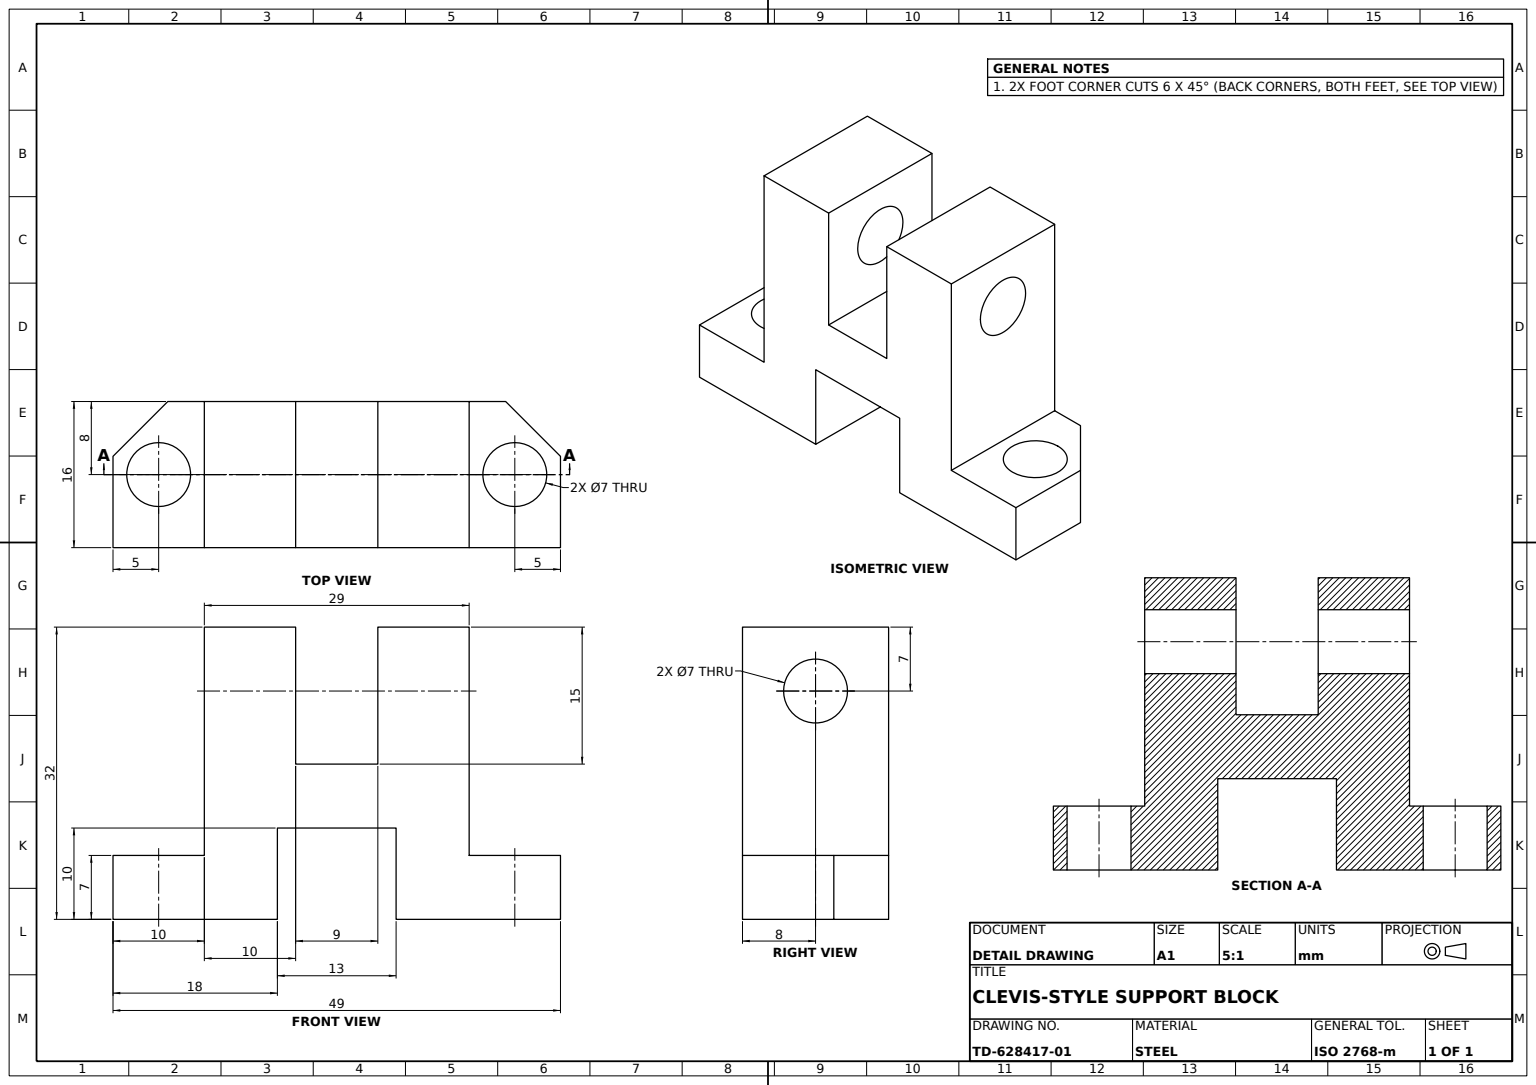
from build123d import *

# Parameters (mm, degrees)
BASE_PROFILE_SKETCH_W     = 29
BASE_PROFILE_SKETCH_H     = 32
BASE_BLOCK_DEPTH          = 16
CENTRE_SLOT_SKETCH_W      = 13
CENTRE_SLOT_SKETCH_H      = 10
CENTRE_SLOT_DEPTH         = 16
SIDE_NOTCH_SKETCH_W       = 9
SIDE_NOTCH_SKETCH_H       = 15
SIDE_NOTCH_DEPTH          = 27.874709301
FOOT_HOLE_SKETCH_R        = 3.5
FOOT_HOLE_DEPTH           = 37.783148315
UPRIGHT_LUG_1_DEPTH       = 7
UPRIGHT_LUG_2_SKETCH_W    = 8
UPRIGHT_LUG_2_SKETCH_H    = 16
UPRIGHT_LUG_2_DEPTH       = 7
LUG_1_CROSS_HOLE_SKETCH_R = 3.5
LUG_1_CROSS_HOLE_DEPTH    = 7
LUG_2_CROSS_HOLE_SKETCH_R = 3.5
LUG_2_CROSS_HOLE_DEPTH    = 7


with BuildPart() as part:
    # Base Profile Sketch → Base Block (new body)
    with BuildSketch(Plane.XY):
        Rectangle(BASE_PROFILE_SKETCH_W, BASE_PROFILE_SKETCH_H)
    extrude(amount=BASE_BLOCK_DEPTH)

    # Centre Slot Sketch → Centre Slot (cut)
    with BuildSketch(Plane.XY.offset(16)):
        with Locations((0, -11)):
            Rectangle(CENTRE_SLOT_SKETCH_W, CENTRE_SLOT_SKETCH_H)
    extrude(amount=-CENTRE_SLOT_DEPTH, mode=Mode.SUBTRACT)

    # Side Notch Sketch → Side Notch (cut, through all)
    with BuildSketch(Plane.XY.offset(16)):
        with Locations((0, 8.5)):
            Rectangle(SIDE_NOTCH_SKETCH_W, SIDE_NOTCH_SKETCH_H)
    extrude(amount=-SIDE_NOTCH_DEPTH, mode=Mode.SUBTRACT)

    # Foot Hole Sketch → Foot Hole (cut, through all)
    with BuildSketch(Plane(origin=(14.5, 0, 0), x_dir=(0, 0, -1), z_dir=(1, 0, 0))):
        with Locations((-8, 9)):
            Circle(FOOT_HOLE_SKETCH_R)
    extrude(amount=-FOOT_HOLE_DEPTH, mode=Mode.SUBTRACT)

    # Upright Lug 1 Sketch → Upright Lug 1 (add)
    with BuildSketch(Plane.XZ.offset(16)):
        Polygon((-18.5, 0), (-24.5, 6), (-24.5, 16), (-14.5, 16), (-6.5, 16), (-6.5, 0), (-14.5, 0), align=None)
    extrude(amount=-UPRIGHT_LUG_1_DEPTH)

    # Upright Lug 2 Sketch → Upright Lug 2 (add)
    with BuildSketch(Plane.XZ.offset(16)):
        Polygon((14.5, 0), (18.5, 0), (24.5, 6), (24.5, 16), (14.5, 16), align=None)
        with Locations((10.5, 8)):
            Rectangle(UPRIGHT_LUG_2_SKETCH_W, UPRIGHT_LUG_2_SKETCH_H)
    extrude(amount=-UPRIGHT_LUG_2_DEPTH)

    # Lug 1 Cross Hole Sketch → Lug 1 Cross Hole (cut)
    with BuildSketch(Plane(origin=(0, -9, 0), x_dir=(1, 0, 0), z_dir=(0, 1, 0))):
        with Locations(Location((-19.5, -8, 0), (0, 0, 270))):
            Circle(LUG_1_CROSS_HOLE_SKETCH_R)
    extrude(amount=-LUG_1_CROSS_HOLE_DEPTH, mode=Mode.SUBTRACT)

    # Lug 2 Cross Hole Sketch → Lug 2 Cross Hole (cut)
    with BuildSketch(Plane(origin=(0, -9, 0), x_dir=(1, 0, 0), z_dir=(0, 1, 0))):
        with Locations(Location((19.5, -8, 0), (0, 0, 270))):
            Circle(LUG_2_CROSS_HOLE_SKETCH_R)
    extrude(amount=-LUG_2_CROSS_HOLE_DEPTH, mode=Mode.SUBTRACT)


solid = part.part
